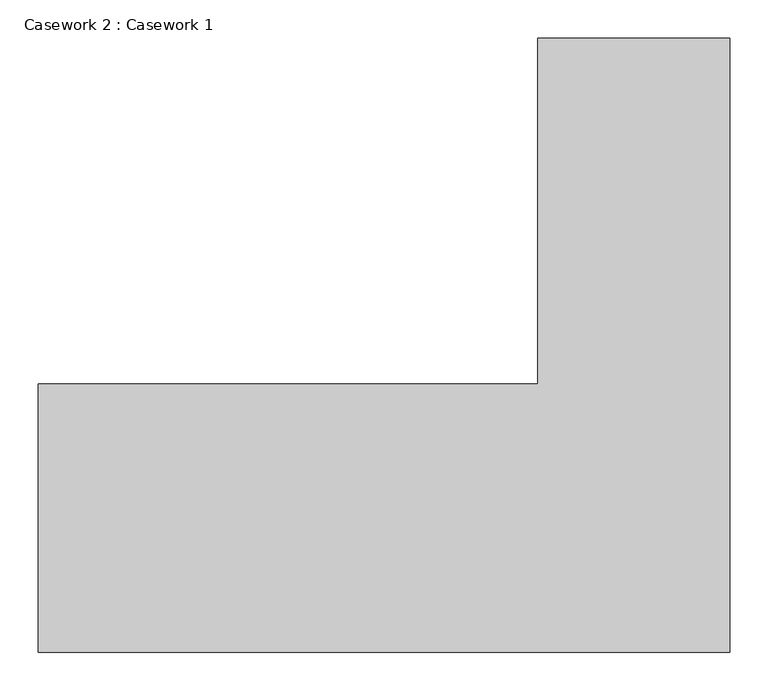
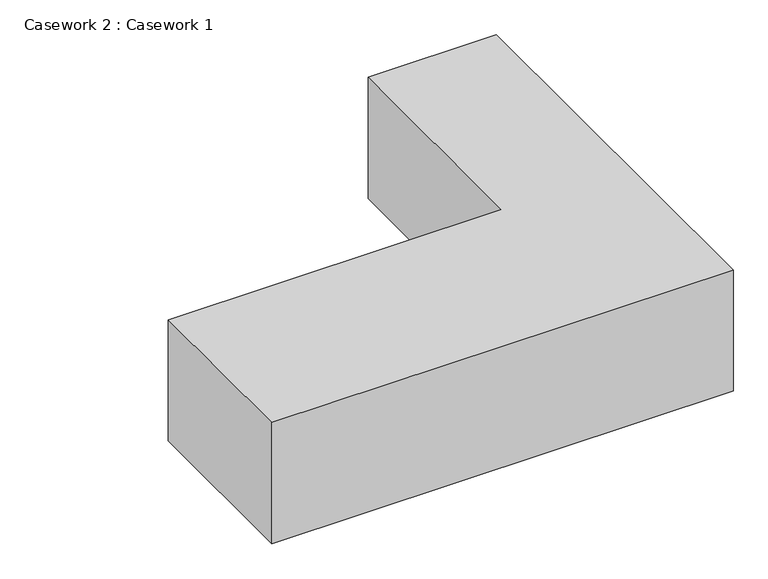
"""IFC4 building model written with IfcOpenShell, lengths in millimetres: furniture geometry, Casework 2 : Casework 1."""

from ifc_helpers import new_model, si_unit, origin, origin_with_axes, place, context, project, spatial, polyline, outline, extrude, source, transform, mapped, element, save


def casework_2_casework_1_9c9d669a(model_context):
    return source(origin(), model_context, "Body", "SweptSolid", [
        extrude(outline(polyline([(23076.1730929, -5475.2269163), (23076.1730929, -6275.2269163), (22176.1730929, -6275.2269163), (22176.1730929, -5925.7891179), (22826.1730929, -5925.7891179), (22826.1730929, -5475.2269163), (23076.1730929, -5475.2269163)])), origin_with_axes(), (0.0, 0.0, 1.0), 250.0),
    ])


if __name__ == "__main__":
    model = new_model("IFC4")
    model_context = context("Model", 3, world=origin())
    ifc_project = project(units=[si_unit("LENGTHUNIT", "METRE", prefix="MILLI")], contexts=[model_context])
    site = spatial("IfcSite", under=ifc_project)
    building = spatial("IfcBuilding", under=site)
    placement = place(None, origin())
    casework_2_casework_1_shape = casework_2_casework_1_9c9d669a(model_context)
    element("IfcFurniture", 1, ObjectType="Casework 2 : Casework 1", at=placement, inside=building, context=model_context, shape_type="MappedRepresentation", body=[
        mapped(casework_2_casework_1_shape, transform((0.0, 0.0, 0.0), x_axis=(1.0, 0.0, 0.0), y_axis=(0.0, 1.0, 0.0), z_axis=(0.0, 0.0, 1.0))),
    ])
    save(model, "model.ifc")
